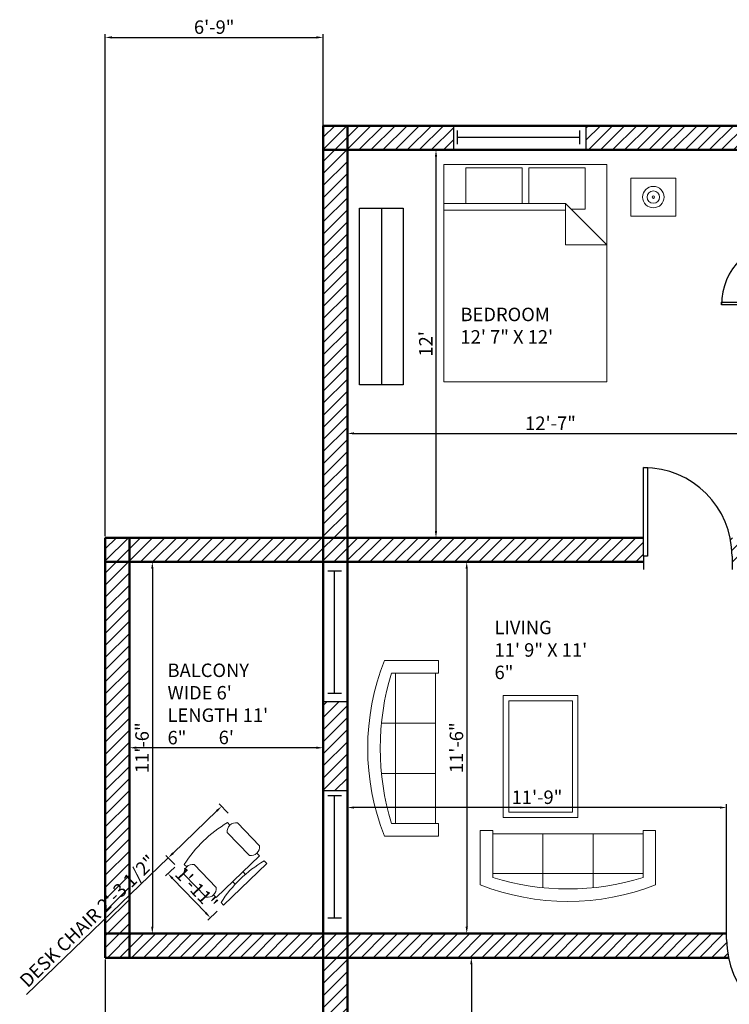
# Model space of a CAD drawing. Units: millimetres. Extents: x 2829 to 4029, y 962 to 1687.
# Tile 6 of 7: x 3412 to 3676, y 1321 to 1687. Entities that reach past the tile are written whole.
import ezdxf

# ---------------------------------------------------------------- set-up
doc = ezdxf.new("R2010")
doc.units = ezdxf.units.MM
for name, color, linetype, lineweight in [('A-ANNO-DIMS', 140, 'Continuous', 18), ('A-AREA-IDEN', 190, 'Continuous', 25), ('A-FLOR-CASE', 90, 'Continuous', 25), ('A-WALL-PATT', 2, 'Continuous', 13), ('doors', 10, 'Continuous', 25), ('furniture', 90, 'Continuous', 18), ('walls', 50, 'Continuous', 50), ('windows', 30, 'Continuous', 25)]:
    doc.layers.add(name, color=color, linetype=linetype, lineweight=lineweight)
doc.styles.get("Standard").update_dxf_attribs({"font": 'arial.ttf'})
doc.dimstyles.new('ISO-25', dxfattribs={"dimtxt": 5, "dimasz": 2.5, "dimexe": 1.25, "dimexo": 0.625, "dimtad": 1, "dimdec": 0, "dimlunit": 3, "dimtxsty": 'Standard', "dimcen": 2.5, "dimadec": 0, "dimazin": 0, "dimtfac": 1, "dimtdec": 0, "dimtmove": 0, "dimatfit": 3, "dimfxl": 1, "dimarcsym": 0})

# ---------------------------------------------------------------- blocks, each defined once
blk = doc.blocks.new('*U2')
for p, q in [((0, 0), (0, -6)), ((40, 0), (40, -6))]:
    blk.add_line(p, q)
blk.add_lwpolyline([(0, 0), (0, 40), (1.75, 40), (1.75, 0)], close=True)
blk.add_arc((0, 0), 40, 0, 90)
blk = doc.blocks.new('*U32')
for p, q in [((0, 4), (0, 0)), ((36, 4), (36, 0)), ((0, 2), (36, 2))]:
    blk.add_line(p, q)
blk = doc.blocks.new('Bed - Queen')
for p, q in [((0, -80.00003), (0, 0)), ((0, 0), (59.99999, 0)), ((59.99999, 0), (59.99999, -80.00003)), ((7.99999, -1.2), (28.79998, -1.2)), ((7.99999, -14.4), (7.99999, -1.2)), ((28.79998, -1.2), (28.79998, -14.4)), ((31.19999, -1.2), (51.99999, -1.2)), ((31.19999, -14.4), (31.19999, -1.2)), ((51.99999, -1.2), (51.99999, -16.4)), ((0, -14.4), (44.8, -14.4)), ((59.99999, -29.6), (44.8, -14.4)), ((44.8, -14.4), (44.8, -29.6)), ((44.8, -16.8), (0, -16.8)), ((51.99999, -16.4), (46.79936, -16.4)), ((44.8, -29.6), (59.99999, -29.6)), ((59.99999, -80.00003), (0, -80.00003))]:
    blk.add_line(p, q)
blk = doc.blocks.new('Sofa - Roundback 7 ft.')
for p, q in [((-12.00002, -32.4421), (-12.00003, -6.5971)), ((11.99997, -32.4421), (11.99998, -6.5971)), ((-36.000027, -34), (-36.000027, -11.4696)), ((-35.999844, -13.3819), (35.9998, -13.3819)), ((35.99998, -34), (35.99998, -11.4696)), ((-36.000027, -32.4421), (35.99998, -32.4421))]:
    blk.add_line(p, q)
for points in [[(-36.000027, -34), (-42.000027, -34), (-42.000027, -8)], [(41.99998, -8), (41.99998, -34), (35.99998, -34)]]:
    blk.add_lwpolyline(points)
for centre, radius, start, end in [((0, -114.25), 114.25, 68.43141, 111.5686), ((-0.00001, -127.1968), 121.1968, 72.72033, 107.2797)]:
    blk.add_arc(centre, radius, start, end)
blk = doc.blocks.new('Chair - Desk')
for p, q in [((-8.5, 0), (-8.5, -1)), ((-8.5, 0), (8.5, 0)), ((8.5, 0), (8.5, -1)), ((-2, -3), (-2, -1.9355)), ((2, -1.9576), (2, -3)), ((-10.5, -5), (-10.5, -14)), ((-8.5, -3), (-8.5, -4)), ((-8.5, -3), (8.5, -3)), ((-6.5, -14), (-6.5, -5)), ((6.5, -5), (6.5, -14)), ((8.5, -3), (8.5, -4)), ((10.5, -14), (10.5, -5)), ((-8.5, -15), (-8.5, -16)), ((8.5, -15), (8.5, -16))]:
    blk.add_line(p, q)
for centre, radius, start, end in [((0, 34.625), 36.625, 256.5803, 283.4197), ((-8.5, -6.5), 2.5, 36.8699, 143.1301), ((8.5, -6.5), 2.5, 36.8699, 143.1301), ((-8.5, -12.5), 2.5, 216.8699, 323.1301), ((0, 19.625), 36.625, 256.5803, 283.4197), ((8.5, -12.5), 2.5, 216.8699, 323.1301)]:
    blk.add_arc(centre, radius, start, end)
blk = doc.blocks.new('*D36')
at = {"layer": 'A-ANNO-DIMS', "color": 0, "lineweight": -2, "transparency": 16777216}
for p, q in [((3533.66, 1539.68), (3533.66, 1531.75)), ((3684.66, 1539.68), (3684.66, 1531.75)), ((3536.16, 1533), (3682.16, 1533))]:
    blk.add_line(p, q, dxfattribs=at)
at = {"layer": 'A-ANNO-DIMS', "color": 0, "transparency": 16777216}
for points in [[(3536.16, 1533.42), (3536.16, 1532.59), (3533.66, 1533)], [(3682.16, 1533.42), (3682.16, 1532.59), (3684.66, 1533)]]:
    blk.add_solid(points, dxfattribs=at)
at = {"layer": 'Defpoints', "color": 0, "transparency": 16777216}
for p in [(3533.66, 1540.3), (3684.66, 1540.3), (3684.66, 1533)]:
    blk.add_point(p, dxfattribs=at)
at = {"layer": 'A-ANNO-DIMS', "color": 0, "transparency": 16777216, "insert": (3609.16, 1536.14), "char_height": 5, "attachment_point": 5}
blk.add_mtext('12\'-7"', dxfattribs=at)
blk = doc.blocks.new('*D37')
at = {"layer": 'A-ANNO-DIMS', "color": 0, "lineweight": -2, "transparency": 16777216}
for p, q in [((3563.74, 1638.27), (3567.84, 1638.27)), ((3566.59, 1635.77), (3566.59, 1496.77)), ((3563.74, 1494.27), (3567.84, 1494.27))]:
    blk.add_line(p, q, dxfattribs=at)
at = {"layer": 'A-ANNO-DIMS', "color": 0, "transparency": 16777216}
for points in [[(3566.17, 1635.77), (3567.01, 1635.77), (3566.59, 1638.27)], [(3566.17, 1496.77), (3567.01, 1496.77), (3566.59, 1494.27)]]:
    blk.add_solid(points, dxfattribs=at)
at = {"layer": 'Defpoints', "color": 0, "transparency": 16777216}
for p in [(3563.12, 1638.27), (3563.12, 1494.27), (3566.59, 1494.27)]:
    blk.add_point(p, dxfattribs=at)
at = {"layer": 'A-ANNO-DIMS', "color": 0, "transparency": 16777216, "insert": (3563.45, 1566.27), "char_height": 5, "attachment_point": 5, "rotation": 90}
blk.add_mtext("12'", dxfattribs=at)
blk = doc.blocks.new('*D47')
at = {"layer": 'A-ANNO-DIMS', "color": 0, "lineweight": -2, "transparency": 16777216}
for p, q in [((3579.16, 1338.27), (3580.98, 1338.27)), ((3579.73, 1335.77), (3579.73, 1196.77)), ((3579.16, 1194.27), (3580.98, 1194.27))]:
    blk.add_line(p, q, dxfattribs=at)
at = {"layer": 'A-ANNO-DIMS', "color": 0, "transparency": 16777216}
for points in [[(3579.31, 1335.77), (3580.15, 1335.77), (3579.73, 1338.27)], [(3579.31, 1196.77), (3580.15, 1196.77), (3579.73, 1194.27)]]:
    blk.add_solid(points, dxfattribs=at)
at = {"layer": 'Defpoints', "color": 0, "transparency": 16777216}
for p in [(3578.53, 1338.27), (3578.53, 1194.27), (3579.73, 1194.27)]:
    blk.add_point(p, dxfattribs=at)
at = {"layer": 'A-ANNO-DIMS', "color": 0, "transparency": 16777216, "insert": (3576.59, 1266.27), "char_height": 5, "attachment_point": 5, "rotation": 90}
blk.add_mtext("12'", dxfattribs=at)
blk = doc.blocks.new('*D49')
at = {"layer": 'A-ANNO-DIMS', "color": 0, "lineweight": -2, "transparency": 16777216}
for p, q in [((3452.66, 1410.61), (3452.66, 1417.52)), ((3522.16, 1416.27), (3455.16, 1416.27)), ((3524.66, 1410.61), (3524.66, 1417.52))]:
    blk.add_line(p, q, dxfattribs=at)
at = {"layer": 'A-ANNO-DIMS', "color": 0, "transparency": 16777216}
for points in [[(3455.16, 1416.69), (3455.16, 1415.85), (3452.66, 1416.27)], [(3522.16, 1416.69), (3522.16, 1415.85), (3524.66, 1416.27)]]:
    blk.add_solid(points, dxfattribs=at)
at = {"layer": 'Defpoints', "color": 0, "transparency": 16777216}
for p in [(3452.66, 1416.27), (3452.66, 1409.99), (3524.66, 1409.99)]:
    blk.add_point(p, dxfattribs=at)
at = {"layer": 'A-ANNO-DIMS', "color": 0, "transparency": 16777216, "insert": (3488.66, 1419.45), "char_height": 5, "attachment_point": 5}
blk.add_mtext("6'", dxfattribs=at)
blk = doc.blocks.new('*D50')
at = {"layer": 'A-ANNO-DIMS', "color": 0, "lineweight": -2, "transparency": 16777216}
for p, q in [((3461.79, 1485.27), (3462.42, 1485.27)), ((3461.17, 1482.77), (3461.17, 1349.77)), ((3461.79, 1347.27), (3462.42, 1347.27))]:
    blk.add_line(p, q, dxfattribs=at)
at = {"layer": 'A-ANNO-DIMS', "color": 0, "transparency": 16777216}
for points in [[(3460.75, 1482.77), (3461.58, 1482.77), (3461.17, 1485.27)], [(3460.75, 1349.77), (3461.58, 1349.77), (3461.17, 1347.27)]]:
    blk.add_solid(points, dxfattribs=at)
at = {"layer": 'Defpoints', "color": 0, "transparency": 16777216}
for p in [(3461.17, 1485.27), (3461.17, 1347.27), (3461.17, 1347.27)]:
    blk.add_point(p, dxfattribs=at)
at = {"layer": 'A-ANNO-DIMS', "color": 0, "transparency": 16777216, "insert": (3457.99, 1416.27), "char_height": 5, "attachment_point": 5, "rotation": 90}
blk.add_mtext('11\'-6"', dxfattribs=at)
blk = doc.blocks.new('*D51')
at = {"layer": 'A-ANNO-DIMS', "color": 0, "lineweight": -2, "transparency": 16777216}
for p, q in [((3576.92, 1485.27), (3579.27, 1485.27)), ((3578.02, 1482.77), (3578.02, 1349.77)), ((3576.92, 1347.27), (3579.27, 1347.27))]:
    blk.add_line(p, q, dxfattribs=at)
at = {"layer": 'A-ANNO-DIMS', "color": 0, "transparency": 16777216}
for points in [[(3577.6, 1482.77), (3578.43, 1482.77), (3578.02, 1485.27)], [(3577.6, 1349.77), (3578.43, 1349.77), (3578.02, 1347.27)]]:
    blk.add_solid(points, dxfattribs=at)
at = {"layer": 'Defpoints', "color": 0, "transparency": 16777216}
for p in [(3576.29, 1485.27), (3576.29, 1347.27), (3578.02, 1347.27)]:
    blk.add_point(p, dxfattribs=at)
at = {"layer": 'A-ANNO-DIMS', "color": 0, "transparency": 16777216, "insert": (3574.84, 1416.27), "char_height": 5, "attachment_point": 5, "rotation": 90}
blk.add_mtext('11\'-6"', dxfattribs=at)
blk = doc.blocks.new('*D52')
at = {"layer": 'A-ANNO-DIMS', "color": 0, "lineweight": -2, "transparency": 16777216}
for p, q in [((3533.66, 1347.9), (3533.66, 1395.32)), ((3672.11, 1394.07), (3536.16, 1394.07)), ((3674.61, 1345.65), (3674.61, 1395.32))]:
    blk.add_line(p, q, dxfattribs=at)
at = {"layer": 'A-ANNO-DIMS', "color": 0, "transparency": 16777216}
for points in [[(3536.16, 1394.48), (3536.16, 1393.65), (3533.66, 1394.07)], [(3672.11, 1394.48), (3672.11, 1393.65), (3674.61, 1394.07)]]:
    blk.add_solid(points, dxfattribs=at)
at = {"layer": 'Defpoints', "color": 0, "transparency": 16777216}
for p in [(3533.66, 1394.07), (3533.66, 1347.27), (3674.61, 1345.02)]:
    blk.add_point(p, dxfattribs=at)
at = {"layer": 'A-ANNO-DIMS', "color": 0, "transparency": 16777216, "insert": (3604.14, 1397.24), "char_height": 5, "attachment_point": 5}
blk.add_mtext('11\'-9"', dxfattribs=at)
blk = doc.blocks.new('*D83')
at = {"layer": 'A-ANNO-DIMS', "color": 0, "lineweight": -2, "transparency": 16777216}
for p, q in [((3489.34, 1391.98), (3486.03, 1395.41)), ((3485.1, 1392.78), (3468.85, 1377.11)), ((3467.05, 1375.37), (3414.45, 1324.64)), ((3469.49, 1372.85), (3466.19, 1376.27))]:
    blk.add_line(p, q, dxfattribs=at)
at = {"layer": 'A-ANNO-DIMS', "color": 0, "transparency": 16777216}
for points in [[(3484.81, 1393.08), (3485.39, 1392.48), (3486.9, 1394.51)], [(3468.56, 1377.41), (3469.14, 1376.81), (3467.05, 1375.37)]]:
    blk.add_solid(points, dxfattribs=at)
at = {"layer": 'Defpoints', "color": 0, "transparency": 16777216}
for p in [(3489.77, 1391.53), (3467.05, 1375.37), (3469.93, 1372.4)]:
    blk.add_point(p, dxfattribs=at)
at = {"layer": 'A-ANNO-DIMS', "color": 0, "transparency": 16777216, "insert": (3437.62, 1351.45), "char_height": 5, "attachment_point": 5, "rotation": 43.9609}
blk.add_mtext('DESK CHAIR 2\'-3 1/2"', dxfattribs=at)
blk = doc.blocks.new('*D84')
at = {"layer": 'A-ANNO-DIMS', "color": 0, "lineweight": -2, "transparency": 16777216}
for p, q in [((3469.48, 1371.96), (3466.05, 1368.66)), ((3468.68, 1367.73), (3481.01, 1354.94)), ((3485.27, 1355.58), (3481.85, 1352.28))]:
    blk.add_line(p, q, dxfattribs=at)
at = {"layer": 'A-ANNO-DIMS', "color": 0, "transparency": 16777216}
for points in [[(3468.98, 1368.02), (3468.38, 1367.44), (3466.95, 1369.53)], [(3481.31, 1355.23), (3480.71, 1354.66), (3482.75, 1353.15)]]:
    blk.add_solid(points, dxfattribs=at)
at = {"layer": 'Defpoints', "color": 0, "transparency": 16777216}
for p in [(3469.93, 1372.4), (3482.75, 1353.15), (3485.72, 1356.02)]:
    blk.add_point(p, dxfattribs=at)
at = {"layer": 'A-ANNO-DIMS', "color": 0, "transparency": 16777216, "insert": (3477.1, 1363.51), "char_height": 5, "attachment_point": 5, "rotation": 313.9609}
blk.add_mtext('1\'-11"', dxfattribs=at)
blk = doc.blocks.new('*D92')
at = {"layer": 'A-ANNO-DIMS', "color": 0, "lineweight": -2, "transparency": 16777216}
for p, q in [((3443.66, 1337.65), (3443.66, 962.22)), ((3991.66, 995.65), (3991.66, 962.22)), ((3446.16, 963.47), (3989.16, 963.47))]:
    blk.add_line(p, q, dxfattribs=at)
at = {"layer": 'A-ANNO-DIMS', "color": 0, "transparency": 16777216}
for points in [[(3446.16, 963.89), (3446.16, 963.05), (3443.66, 963.47)], [(3989.16, 963.89), (3989.16, 963.05), (3991.66, 963.47)]]:
    blk.add_solid(points, dxfattribs=at)
at = {"layer": 'Defpoints', "color": 0, "transparency": 16777216}
for p in [(3443.66, 1338.27), (3991.66, 996.27), (3991.66, 963.47)]:
    blk.add_point(p, dxfattribs=at)
at = {"layer": 'A-ANNO-DIMS', "color": 0, "transparency": 16777216, "insert": (3717.66, 966.65), "char_height": 5, "attachment_point": 5}
blk.add_mtext('45\'-8"', dxfattribs=at)
blk = doc.blocks.new('*D94')
at = {"layer": 'A-ANNO-DIMS', "color": 0, "lineweight": -2, "transparency": 16777216}
for p, q in [((3443.66, 1494.9), (3443.66, 1681.32)), ((3446.16, 1680.07), (3522.16, 1680.07)), ((3524.66, 1494.9), (3524.66, 1681.32))]:
    blk.add_line(p, q, dxfattribs=at)
at = {"layer": 'A-ANNO-DIMS', "color": 0, "transparency": 16777216}
for points in [[(3446.16, 1680.49), (3446.16, 1679.65), (3443.66, 1680.07)], [(3522.16, 1680.49), (3522.16, 1679.65), (3524.66, 1680.07)]]:
    blk.add_solid(points, dxfattribs=at)
at = {"layer": 'Defpoints', "color": 0, "transparency": 16777216}
for p in [(3524.66, 1680.07), (3443.66, 1494.27), (3524.66, 1494.27)]:
    blk.add_point(p, dxfattribs=at)
at = {"layer": 'A-ANNO-DIMS', "color": 0, "transparency": 16777216, "insert": (3484.16, 1683.25), "char_height": 5, "attachment_point": 5}
blk.add_mtext('6\'-9"', dxfattribs=at)

msp = doc.modelspace()

# ---------------------------------------------------------------- hatches: boundary and pattern name
at = {"layer": 'A-WALL-PATT'}
h = msp.add_hatch(dxfattribs=at)
h.set_pattern_fill('ANSI31', color=256)
h.set_pattern_definition([(45, (-1090.0668, 570.9627), (-2.245064, 2.245064), [])])
h.paths.add_polyline_path([(3524.66, 1494.27), (3452.66, 1494.27), (3452.66, 1485.27), (3524.66, 1485.27)])
h.paths.add_polyline_path([(3452.66, 1494.27), (3443.66, 1494.27), (3443.66, 1485.27), (3452.66, 1485.27)])
h.paths.add_polyline_path([(3452.66, 1485.27), (3443.66, 1485.27), (3443.66, 1347.27), (3452.66, 1347.27)])
h.paths.add_polyline_path([(3533.66, 1433.28), (3524.66, 1433.28), (3524.66, 1400.41), (3533.66, 1400.41)])
h.paths.add_polyline_path([(3524.66, 1347.27), (3452.66, 1347.27), (3452.66, 1338.27), (3524.66, 1338.27)])
h.paths.add_polyline_path([(3452.66, 1347.27), (3443.66, 1347.27), (3443.66, 1338.27), (3452.66, 1338.27)])
h.paths.add_polyline_path([(3533.66, 1347.27), (3524.66, 1347.27), (3524.66, 1338.27), (3533.66, 1338.27)])
h.paths.add_polyline_path([(3674.61, 1345.02), (3674.61, 1347.27), (3533.66, 1347.27), (3533.66, 1338.27), (3675.31, 1338.27, -0.051672)])
h.paths.add_polyline_path([(3533.66, 1638.27), (3524.66, 1638.27), (3524.66, 1494.27), (3533.66, 1494.27)])
h.paths.add_polyline_path([(3533.66, 1494.27), (3524.66, 1494.27), (3524.66, 1485.27), (3533.66, 1485.27)])
h.paths.add_polyline_path([(3643.72, 1494.27), (3533.66, 1494.27), (3533.66, 1485.27), (3643.72, 1485.27), (3643.72, 1487.41)])
h.paths.add_polyline_path([(3533.66, 1647.27), (3524.66, 1647.27), (3524.66, 1638.27), (3533.66, 1638.27)])
h.paths.add_polyline_path([(3573.07, 1647.27), (3533.66, 1647.27), (3533.66, 1638.27), (3573.07, 1638.27)])
h.paths.add_polyline_path([(3684.66, 1647.27), (3622.32, 1647.27), (3622.32, 1638.27), (3684.66, 1638.27)])
h.paths.add_polyline_path([(3693.66, 1647.27), (3684.66, 1647.27), (3684.66, 1638.27), (3693.66, 1638.27)])
h.paths.add_polyline_path([(3693.66, 1638.27), (3684.66, 1638.27), (3684.66, 1601.42, -0.100401), (3693.66, 1604.42)])
h.paths.add_polyline_path([(3693.66, 1580.73), (3684.66, 1580.73), (3684.66, 1542.27), (3693.66, 1542.27)])
h.paths.add_polyline_path([(3693.66, 1542.27), (3684.66, 1542.27), (3684.66, 1533.27), (3693.66, 1533.27)])
h.paths.add_polyline_path([(3693.66, 1533.27), (3684.66, 1533.27), (3684.66, 1494.27), (3693.66, 1494.27)])
h.paths.add_polyline_path([(3693.66, 1494.27), (3684.66, 1494.27), (3684.66, 1485.27), (3693.66, 1485.27)])
h.paths.add_polyline_path([(3684.66, 1494.27), (3675.91, 1494.27, -0.052559), (3676.64, 1487.41), (3676.64, 1485.27), (3684.66, 1485.27)])
h.paths.add_polyline_path([(3753.66, 1542.27), (3693.66, 1542.27), (3693.66, 1533.27), (3753.66, 1533.27)])
h.paths.add_polyline_path([(3762.66, 1542.27), (3753.66, 1542.27), (3753.66, 1533.27), (3762.66, 1533.27)])
h.paths.add_polyline_path([(3762.66, 1638.27), (3753.66, 1638.27), (3753.66, 1542.27), (3762.66, 1542.27)])
h.paths.add_polyline_path([(3762.66, 1647.27), (3753.66, 1647.27), (3753.66, 1638.27), (3762.66, 1638.27)])
h.paths.add_polyline_path([(3753.66, 1647.27), (3733.82, 1647.27), (3733.82, 1638.27), (3753.66, 1638.27)])
h.paths.add_polyline_path([(3706.41, 1647.27), (3693.66, 1647.27), (3693.66, 1638.27), (3706.41, 1638.27)])
h.paths.add_polyline_path([(3822.66, 1647.27), (3804.07, 1647.27), (3804.07, 1638.27), (3822.66, 1638.27)])
h.paths.add_polyline_path([(3778.61, 1647.27), (3762.66, 1647.27), (3762.66, 1638.27), (3778.61, 1638.27)])
h.paths.add_polyline_path([(3822.66, 1542.27), (3762.66, 1542.27), (3762.66, 1533.27), (3822.66, 1533.27)])
h.paths.add_polyline_path([(3831.66, 1542.27), (3822.66, 1542.27), (3822.66, 1533.27), (3831.66, 1533.27)])
h.paths.add_polyline_path([(3831.66, 1587.4), (3822.66, 1587.4), (3822.66, 1542.27), (3831.66, 1542.27)])
h.paths.add_polyline_path([(3831.66, 1638.27), (3822.66, 1638.27), (3822.66, 1611.22, -0.098322), (3831.66, 1608.9)])
h.paths.add_polyline_path([(3831.66, 1647.27), (3822.66, 1647.27), (3822.66, 1638.27), (3831.66, 1638.27)])
h.paths.add_polyline_path([(3883.77, 1647.27), (3831.66, 1647.27), (3831.66, 1638.27), (3883.77, 1638.27)])
h.paths.add_polyline_path([(3982.66, 1647.27), (3934.96, 1647.27), (3934.96, 1638.27), (3982.66, 1638.27)])
h.paths.add_polyline_path([(3991.66, 1647.27), (3982.66, 1647.27), (3982.66, 1638.27), (3991.66, 1638.27)])
h.paths.add_polyline_path([(3991.66, 1638.27), (3982.66, 1638.27), (3982.66, 1494.27), (3991.66, 1494.27)])
h.paths.add_polyline_path([(3991.66, 1494.27), (3982.66, 1494.27), (3982.66, 1485.27), (3991.66, 1485.27)])
h.paths.add_polyline_path([(3982.66, 1494.27), (3831.66, 1494.27), (3831.66, 1485.27), (3982.66, 1485.27)])
h.paths.add_polyline_path([(3831.66, 1494.27), (3822.66, 1494.27), (3822.66, 1485.27), (3831.66, 1485.27)])
h.paths.add_polyline_path([(3991.66, 1485.27), (3982.66, 1485.27), (3982.66, 1463.05, -0.057246), (3990.12, 1463.9), (3991.66, 1463.9)])
h.paths.add_polyline_path([(3991.66, 1430.98), (3990.12, 1430.98), (3982.66, 1430.98), (3982.66, 1347.27), (3991.66, 1347.27)])
h.paths.add_polyline_path([(3982.66, 1347.27), (3786.66, 1347.27), (3786.66, 1338.27), (3982.66, 1338.27)])
h.paths.add_polyline_path([(3991.66, 1347.27), (3982.66, 1347.27), (3982.66, 1338.27), (3991.66, 1338.27)])
h.paths.add_polyline_path([(3991.66, 1338.27), (3982.66, 1338.27), (3982.66, 1005.27), (3991.66, 1005.27)])
h.paths.add_polyline_path([(3982.66, 1194.27), (3879.62, 1194.27), (3879.62, 1185.27), (3982.66, 1185.27)])
h.paths.add_polyline_path([(3853.79, 1194.27), (3795.66, 1194.27), (3795.66, 1185.27), (3853.79, 1185.27)])
h.paths.add_polyline_path([(3795.66, 1194.27), (3786.66, 1194.27), (3786.66, 1185.27), (3795.66, 1185.27)])
h.paths.add_polyline_path([(3795.66, 1290.27), (3786.66, 1290.27), (3786.66, 1194.27), (3795.66, 1194.27)])
h.paths.add_polyline_path([(3726.66, 1230.69), (3717.66, 1230.69), (3717.66, 1194.27), (3726.66, 1194.27)])
h.paths.add_polyline_path([(3726.66, 1194.27), (3717.66, 1194.27), (3717.66, 1185.27), (3726.66, 1185.27)])
h.paths.add_polyline_path([(3742.53, 1194.27), (3726.66, 1194.27), (3726.66, 1185.27), (3742.53, 1185.27)])
h.paths.add_polyline_path([(3786.66, 1194.27), (3767.92, 1194.27), (3767.92, 1185.27), (3786.66, 1185.27)])
h.paths.add_polyline_path([(3726.66, 1290.27), (3717.66, 1290.27), (3717.66, 1252.42, -0.097806), (3726.66, 1254.54)])
h.paths.add_polyline_path([(3726.66, 1299.27), (3717.66, 1299.27), (3717.66, 1290.27), (3726.66, 1290.27)])
h.paths.add_polyline_path([(3786.66, 1299.27), (3726.66, 1299.27), (3726.66, 1290.27), (3786.66, 1290.27)])
h.paths.add_polyline_path([(3795.66, 1299.27), (3786.66, 1299.27), (3786.66, 1290.27), (3795.66, 1290.27)])
h.paths.add_polyline_path([(3726.66, 1338.27), (3717.66, 1338.27), (3717.66, 1299.27), (3726.66, 1299.27)])
h.paths.add_polyline_path([(3717.66, 1194.27), (3641.7, 1194.27), (3641.7, 1185.27), (3717.66, 1185.27)])
h.paths.add_polyline_path([(3588.68, 1194.27), (3533.66, 1194.27), (3533.66, 1185.27), (3588.68, 1185.27)])
h.paths.add_polyline_path([(3533.66, 1194.27), (3524.66, 1194.27), (3524.66, 1185.27), (3533.66, 1185.27)])
h.paths.add_polyline_path([(3533.66, 1338.27), (3524.66, 1338.27), (3524.66, 1194.27), (3533.66, 1194.27)])
h.paths.add_polyline_path([(3533.66, 1185.27), (3524.66, 1185.27), (3524.66, 1005.27), (3533.66, 1005.27)])
h.paths.add_polyline_path([(3717.66, 1005.27), (3533.66, 1005.27), (3533.66, 996.27), (3717.66, 996.27)])
h.paths.add_polyline_path([(3726.66, 1005.27), (3717.66, 1005.27), (3717.66, 996.27), (3726.66, 996.27)])
h.paths.add_polyline_path([(3533.66, 1005.27), (3524.66, 1005.27), (3524.66, 996.27), (3533.66, 996.27)])
h.paths.add_polyline_path([(3786.66, 1005.27), (3726.66, 1005.27), (3726.66, 996.27), (3786.66, 996.27)])
h.paths.add_polyline_path([(3982.66, 1005.27), (3795.66, 1005.27), (3795.66, 996.27), (3982.66, 996.27)])
h.paths.add_polyline_path([(3795.66, 1005.27), (3786.66, 1005.27), (3786.66, 996.27), (3795.66, 996.27)])
h.paths.add_polyline_path([(3991.66, 1005.27), (3982.66, 1005.27), (3982.66, 996.27), (3991.66, 996.27)])

# ---------------------------------------------------------------- linework, layer by layer
at = {"layer": 'A-FLOR-CASE'}
msp.add_line((3546.32, 1616.66), (3546.32, 1551.06), dxfattribs=at)
msp.add_lwpolyline([(3538.19, 1616.66), (3554.45, 1616.66), (3554.45, 1551.06), (3538.19, 1551.06)], close=True, dxfattribs=at)
at = {"layer": 'furniture'}
for points in [[(3638.97, 1627.85), (3655.78, 1627.85), (3655.78, 1613.7), (3638.97, 1613.7)], [(3591.62, 1435.71), (3619.36, 1435.71), (3619.36, 1390.4), (3591.62, 1390.4)], [(3593.62, 1433.71), (3617.36, 1433.71), (3617.36, 1392.4), (3593.62, 1392.4)]]:
    msp.add_lwpolyline(points, close=True, dxfattribs=at)
for radius in [3.99, 2.31, 0.47]:
    msp.add_circle((3647.38, 1620.77), radius, dxfattribs=at)
at = {"layer": 'walls'}
for p, q in [((3524.66, 1647.27), (3524.66, 996.27)), ((3524.66, 1647.27), (3991.66, 1647.27)), ((3533.66, 1647.27), (3533.66, 996.27)), ((3524.66, 1638.27), (3991.66, 1638.27)), ((3443.66, 1494.27), (3643.72, 1494.27)), ((3443.66, 1494.27), (3443.66, 1338.27)), ((3452.66, 1494.27), (3452.66, 1338.27)), ((3524.66, 1494.27), (3643.72, 1494.27)), ((3443.66, 1485.27), (3643.72, 1485.27)), ((3524.66, 1485.27), (3643.72, 1485.27)), ((3443.66, 1347.27), (3533.66, 1347.27)), ((3443.66, 1347.27), (3674.61, 1347.27)), ((3443.66, 1338.27), (3533.66, 1338.27)), ((3443.66, 1338.27), (3675.31, 1338.27))]:
    msp.add_line(p, q, dxfattribs=at)
at = {"layer": 'windows'}
for p, q in [((3573.07, 1647.27), (3573.07, 1638.27)), ((3622.32, 1647.27), (3622.32, 1638.27)), ((3533.66, 1433.28), (3524.66, 1433.28)), ((3524.66, 1400.41), (3533.66, 1400.41))]:
    msp.add_line(p, q, dxfattribs=at)

# ---------------------------------------------------------------- block references
at = {"layer": 'doors'}
for p, xscale, yscale, zscale, rotation in [((3696.56, 1580.73), 0.5965458762151612, 0.5965458762151612, 0.5965458762151612, 90), ((3707.53, 1345.02), 0.8229573665348725, 0.8229573665348725, 0.8229573665348725, 180)]:
    msp.add_blockref('*U2', p, dxfattribs=dict(at, xscale=xscale, yscale=yscale, zscale=zscale, rotation=rotation))
at = {"layer": 'doors', "xscale": 0.8229573665348725, "yscale": 0.8229573665348725, "zscale": 0.8229573665348725}
msp.add_blockref('*U2', (3643.72, 1487.41), dxfattribs=at)
at = {"layer": 'furniture', "xscale": 1.009641765202986, "yscale": 1.009641765202986, "zscale": 1.009641765202986}
msp.add_blockref('Bed - Queen', (3569.55, 1632.88), dxfattribs=at)
at = {"layer": 'furniture'}
for name, p, xscale, yscale, zscale, rotation in [('Sofa - Roundback 7 ft.', (3541.2, 1416.06), 0.7756069155116014, 0.7756069155116014, 0.7756069155116014, 89.99999999999999), ('Chair - Desk', (3495.64, 1365.59), 1.312866679139032, 1.312866679139032, 1.312866679139032, 223.9609120105676), ('Sofa - Roundback 7 ft.', (3615.64, 1359.17), 0.7756069155116014, 0.7756069155116014, 0.7756069155116014, 180)]:
    msp.add_blockref(name, p, dxfattribs=dict(at, xscale=xscale, yscale=yscale, zscale=zscale, rotation=rotation))
at = {"layer": 'windows', "xscale": 1.262484112988456, "yscale": 1.262484112988456, "zscale": 1.262484112988456}
msp.add_blockref('*U32', (3574.43, 1640.47), dxfattribs=at)
at = {"layer": 'windows', "xscale": 1.262484112988456, "yscale": 1.262484112988456, "zscale": 1.262484112988456, "rotation": 90}
for p in [(3531.43, 1436.55), (3531.43, 1353.14)]:
    msp.add_blockref('*U32', p, dxfattribs=at)

# ---------------------------------------------------------------- texts
at = {"layer": 'A-AREA-IDEN', "char_height": 5, "attachment_point": 1}
for s, width, insert in [('BEDROOM\\P12\' 7" X 12\'', 54.4423, (3575.69, 1579.69)), ('LIVING\\P11\' 9" X 11\' 6"', 38.671, (3588.35, 1463.42)), ('BALCONY\\PWIDE 6\'\\PLENGTH 11\' 6"', 42.1472, (3466.82, 1447.53))]:
    msp.add_mtext_dynamic_manual_height_columns(s, width=width, gutter_width=12.5, heights=[0], dxfattribs=dict(at, insert=insert))

# ---------------------------------------------------------------- dimensions: what is measured, and where the dimension line sits
at = {"layer": 'A-ANNO-DIMS'}
for base, p1, p2, override, picture, middle in [((3524.66, 1680.07), (3443.66, 1494.27), (3524.66, 1494.27), {"dimdec": 1, "dimlfac": 1, "dimrnd": 0, "dimzin": 1, "dimdsep": 46, "dimlunit": 4, "dimfrac": 2}, '*D94', (3484.16, 1683.25)), ((3684.66, 1533), (3533.66, 1540.3), (3684.66, 1540.3), {"dimclrd": 0, "dimclre": 0, "dimclrt": 0}, '*D36', (3609.16, 1536.14)), ((3452.66, 1416.27), (3524.66, 1409.99), (3452.66, 1409.99), {"dimclrd": 0, "dimclre": 0, "dimclrt": 0}, '*D49', (3488.66, 1419.45)), ((3533.66, 1394.07), (3674.61, 1345.02), (3533.66, 1347.27), {"dimclrd": 0, "dimclre": 0, "dimclrt": 0}, '*D52', (3604.14, 1397.24)), ((3991.66, 963.47), (3443.66, 1338.27), (3991.66, 996.27), {"dimdec": 1, "dimlfac": 1, "dimrnd": 0, "dimzin": 1, "dimdsep": 46, "dimlunit": 4, "dimfrac": 2}, '*D92', (3717.66, 966.65))]:
    dim = msp.add_linear_dim(base=base, p1=p1, p2=p2, dimstyle='ISO-25', override=override, dxfattribs=at)
    dim.commit()
    dim.dimension.update_dxf_attribs({"geometry": picture, "text_midpoint": middle})
for base, p1, p2, angle, override, picture, middle in [((3566.59, 1494.27), (3563.12, 1638.27), (3563.12, 1494.27), 90, {"dimclrd": 0, "dimclre": 0, "dimclrt": 0}, '*D37', (3563.45, 1566.27)), ((3461.17, 1347.27), (3461.17, 1485.27), (3461.17, 1347.27), 90, {"dimclrd": 0, "dimclre": 0, "dimclrt": 0}, '*D50', (3457.99, 1416.27)), ((3578.02, 1347.27), (3576.29, 1485.27), (3576.29, 1347.27), 90, {"dimclrd": 0, "dimclre": 0, "dimclrt": 0}, '*D51', (3574.84, 1416.27)), ((3482.75, 1353.15), (3469.93, 1372.4), (3485.72, 1356.02), 313.9609, {"dimdec": 1, "dimlfac": 1, "dimrnd": 0, "dimzin": 1, "dimdsep": 46, "dimlunit": 4, "dimfrac": 2}, '*D84', (3477.1, 1363.51)), ((3579.73, 1194.27), (3578.53, 1338.27), (3578.53, 1194.27), 90, {"dimclrd": 0, "dimclre": 0, "dimclrt": 0}, '*D47', (3576.59, 1266.27))]:
    dim = msp.add_linear_dim(base=base, p1=p1, p2=p2, angle=angle, dimstyle='ISO-25', override=override, dxfattribs=at)
    dim.commit()
    dim.dimension.update_dxf_attribs({"geometry": picture, "text_midpoint": middle})
dim = msp.add_linear_dim(base=(3467.05, 1375.37), p1=(3489.77, 1391.53), p2=(3469.93, 1372.4), angle=223.9609, text='DESK CHAIR <>', dimstyle='ISO-25', override={"dimdec": 1, "dimlfac": 1, "dimrnd": 0, "dimzin": 1, "dimdsep": 46, "dimlunit": 4, "dimfrac": 2}, dxfattribs=at)
dim.commit()
dim.dimension.update_dxf_attribs({"geometry": '*D83', "text_midpoint": (3437.62, 1351.45)})

doc.saveas('drawing.dxf')
